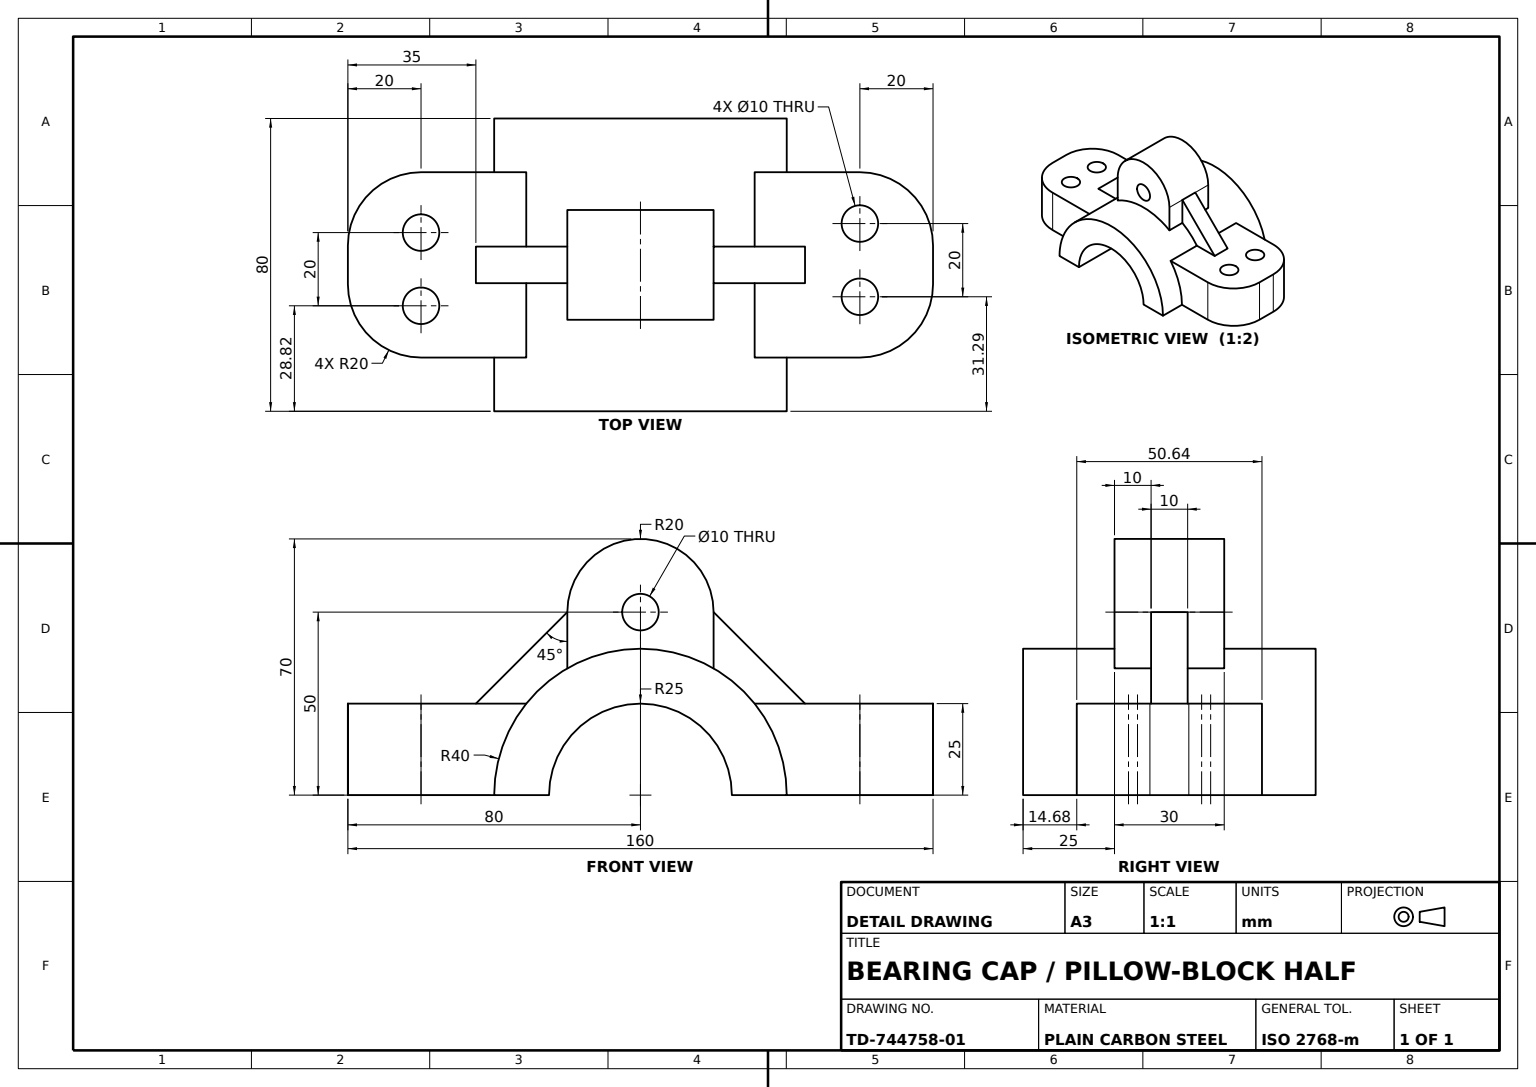
from build123d import *

# Parameters (mm, degrees)
HOUSING_BLOCK_DEPTH           = 40
TOP_LUG_SKETCH_R              = 5
TOP_LUG_DEPTH                 = 15
BASE_FLANGE_SKETCH_W          = 70
BASE_FLANGE_SKETCH_H          = 50.64236497
BASE_FLANGE_DEPTH             = 25
BEARING_SEAT_CUT_DEPTH        = 80
FLANGE_END_ROUND_R20_A_R      = 20
FLANGE_END_ROUND_R20_B_R      = 20
MOUNTING_HOLES_SET_1_SKETCH_R = 5
MOUNTING_HOLES_SET_1_DEPTH    = 25
MOUNTING_HOLES_SET_2_SKETCH_R = 5
MOUNTING_HOLES_SET_2_DEPTH    = 25
SUPPORT_RIB_1_REACH           = 115.578
SUPPORT_RIB_1_SKETCH_WALL_W   = 264.511672892
SUPPORT_RIB_1_SKETCH_WALL_H   = 10
SUPPORT_RIB_2_REACH           = 115.578
SUPPORT_RIB_2_SKETCH_WALL_W   = 264.511672892
SUPPORT_RIB_2_SKETCH_WALL_H   = 10


with BuildPart() as part:
    # Housing Block Sketch → Housing Block (new, symmetric)
    with BuildSketch(Plane.XY):
        with BuildLine():
            Line((-40, 0), (-25, 0))
            ThreePointArc((-25, 0), (0, 25), (25, 0))
            Line((25, 0), (40, 0))
            ThreePointArc((40, 0), (0, 40), (-40, 0))
        make_face()
    extrude(amount=HOUSING_BLOCK_DEPTH, both=True)

    # Top Lug Sketch → Top Lug (add, symmetric)
    with BuildSketch(Plane.XY):
        with BuildLine():
            Line((-20, 50), (-20, 34.002392221))
            Line((-20, 34.002392221), (20, 34.641016151))
            Line((20, 34.641016151), (20, 50))
            ThreePointArc((20, 50), (0, 70), (-20, 50))
        make_face()
        with Locations((0, 50)):
            Circle(TOP_LUG_SKETCH_R, mode=Mode.SUBTRACT)
    extrude(amount=TOP_LUG_DEPTH, both=True)

    # Base Flange Sketch → Base Flange (add)
    with BuildSketch(Plane(origin=(0, 0, 0), x_dir=(1, 0, 0), z_dir=(0, 1, 0))):
        with Locations((45, 0)):
            Rectangle(BASE_FLANGE_SKETCH_W, BASE_FLANGE_SKETCH_H)
        with Locations((-45, 0)):
            Rectangle(BASE_FLANGE_SKETCH_W, BASE_FLANGE_SKETCH_H)
    extrude(amount=BASE_FLANGE_DEPTH)

    # Bearing Seat Sketch → Bearing Seat Cut (cut)
    with BuildSketch(Plane.XY.offset(25.321182485)):
        with BuildLine():
            Line((-10, 22.912878475), (-10, 0))
            Line((-10, 0), (-25, 0))
            ThreePointArc((-25, 0), (-20.916500663, 13.693063938), (-10, 22.912878475))
        make_face()
        with BuildLine():
            Line((10, 22.912878475), (10, 0))
            Line((10, 0), (25, 0))
            ThreePointArc((25, 0), (20.916500663, 13.693063938), (10, 22.912878475))
        make_face()
    extrude(amount=-BEARING_SEAT_CUT_DEPTH, mode=Mode.SUBTRACT)

    # Flange End Round R20 A
    flange_end_round_r20_a_edges = [part.edges().sort_by_distance(p)[0] for p in [
        (80, 12.5, -25.321182485),
        (80, 12.5, 25.321182485),
        (-80, 12.5, 25.321182485),
    ]]
    fillet(flange_end_round_r20_a_edges, radius=FLANGE_END_ROUND_R20_A_R)

    # Flange End Round R20 B
    flange_end_round_r20_b_edges = [part.edges().sort_by_distance(p)[0] for p in [
        (-80, 12.5, -25.321182485),
    ]]
    fillet(flange_end_round_r20_b_edges, radius=FLANGE_END_ROUND_R20_B_R)

    # Mounting Holes Set 1 Sketch → Mounting Holes Set 1 (cut)
    with BuildSketch(Plane(origin=(0, 25, 0), x_dir=(1, 0, 0), z_dir=(0, 1, 0))):
        with Locations(Location((-60, 8.824452572, 0), (0, 0, 270))):
            Circle(MOUNTING_HOLES_SET_1_SKETCH_R)
        with Locations(Location((-60, -11.175547428, 0), (0, 0, 270))):
            Circle(MOUNTING_HOLES_SET_1_SKETCH_R)
    extrude(amount=-MOUNTING_HOLES_SET_1_DEPTH, mode=Mode.SUBTRACT)

    # Mounting Holes Set 2 Sketch → Mounting Holes Set 2 (cut)
    with BuildSketch(Plane(origin=(0, 25, 0), x_dir=(1, 0, 0), z_dir=(0, 1, 0))):
        with Locations(Location((60, 11.288668944, 0), (0, 0, 270))):
            Circle(MOUNTING_HOLES_SET_2_SKETCH_R)
        with Locations(Location((60, -8.711331056, 0), (0, 0, 270))):
            Circle(MOUNTING_HOLES_SET_2_SKETCH_R)
    extrude(amount=-MOUNTING_HOLES_SET_2_DEPTH, mode=Mode.SUBTRACT)

    # Support Rib 1 Sketch wall → Support Rib 1 (add, up to next)
    with BuildSketch(Plane(origin=(-32.5, 37.5, 0), x_dir=(-0.707106781187, -0.707106781187, 0), z_dir=(0.707106781187, -0.707106781187, 0)), mode=Mode.PRIVATE) as support_rib_1_sk1:
        Rectangle(SUPPORT_RIB_1_SKETCH_WALL_W, SUPPORT_RIB_1_SKETCH_WALL_H)
    support_rib_1_tool1 = extrude(support_rib_1_sk1.sketch, amount=SUPPORT_RIB_1_REACH, mode=Mode.PRIVATE) - part.part
    add(support_rib_1_tool1.solids().sort_by_distance((-32.5, 37.5, 0))[0])

    # Support Rib 2 Sketch wall → Support Rib 2 (add, up to next)
    with BuildSketch(Plane(origin=(32.5, 37.5, 0), x_dir=(0.707106781187, -0.707106781187, 0), z_dir=(0.707106781187, 0.707106781187, 0)), mode=Mode.PRIVATE) as support_rib_2_sk1:
        Rectangle(SUPPORT_RIB_2_SKETCH_WALL_W, SUPPORT_RIB_2_SKETCH_WALL_H)
    support_rib_2_tool1 = extrude(support_rib_2_sk1.sketch, amount=-SUPPORT_RIB_2_REACH, mode=Mode.PRIVATE) - part.part
    add(support_rib_2_tool1.solids().sort_by_distance((32.5, 37.5, 0))[0])


solid = part.part
